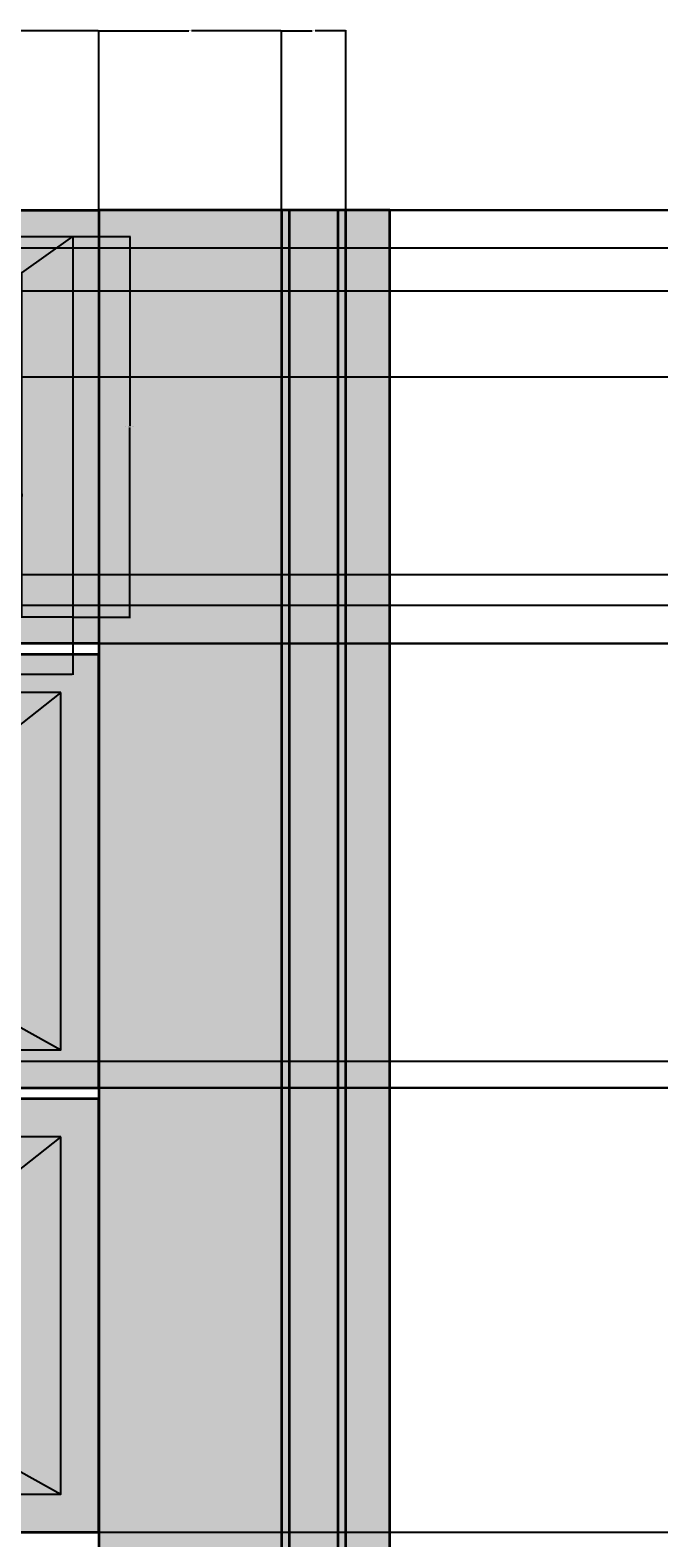
# Model space of a CAD drawing. Units: feet. Extents: x 1141 to 2858, y 751 to 1654.
# Tile 8 of 13: x 2096 to 2288, y 1195 to 1654. Entities that reach past the tile are written whole.
import ezdxf

# ---------------------------------------------------------------- set-up
doc = ezdxf.new("R2010")
doc.units = ezdxf.units.FT
for name, color, linetype, lineweight in [('A-ANNO-DIMS', 2, 'Continuous', 18), ('A-ELEV', 7, 'Continuous', 35), ('A-ELEV-PATT', 8, 'Continuous', 13), ('A-GLAZ', 4, 'Continuous', 25)]:
    doc.layers.add(name, color=color, linetype=linetype, lineweight=lineweight)
doc.styles.get("Standard").update_dxf_attribs({"font": 'arial.ttf'})
doc.dimstyles.get("Standard").update_dxf_attribs({"dimtxt": 0.18, "dimasz": 0.18, "dimexe": 0.18, "dimexo": 0.0625, "dimgap": 0.09, "dimtad": 0, "dimtih": 1, "dimtoh": 1, "dimdec": 1, "dimzin": 0, "dimdsep": 46, "dimlunit": 3, "dimtxsty": 'Standard', "dimcen": 0.09, "dimadec": 0, "dimazin": 0, "dimtfac": 1, "dimtdec": 1, "dimtofl": 0, "dimtmove": 0, "dimatfit": 3, "dimfxl": 1, "dimtolj": 1, "dimtzin": 0, "dimarcsym": 0})

# ---------------------------------------------------------------- blocks, each defined once
blk = doc.blocks.new('WIN-SIDE-A')
blk.add_line((63.09, 104.94), (78.57, 116.03))
blk.add_line((63.09, 104.94), (78.57, 116.03))
for points in [[(78.57, 0), (0, 0), (0, 116.03), (78.57, 116.03)], [(78.57, 0), (0, 0), (0, 116.03), (78.57, 116.03)], [(31.54, 104.94), (32.46, 104.94), (32.46, 0), (31.54, 0)], [(0, 37.61), (63.09, 37.61), (63.09, 36.79), (0, 36.79)]]:
    blk.add_lwpolyline(points, close=True)
for points in [[(63.09, 0), (63.09, 104.94), (0, 104.94)], [(63.09, 0), (63.09, 104.94), (0, 104.94)], [(31.54, 37.61), (31.54, 104.94), (32.46, 104.94), (32.46, 37.61)], [(31.54, 36.79), (0, 36.79), (0, 37.61), (31.54, 37.61)], [(32.46, 36.79), (32.46, 0), (31.54, 0), (31.54, 36.79)], [(32.46, 37.61), (63.09, 37.61), (63.09, 36.79), (32.46, 36.79)]]:
    blk.add_lwpolyline(points)
blk = doc.blocks.new('BALCONY-GLAZ-A')
for p, q in [((0, 108.84), (16.63, 95.74)), ((0, 108.84), (16.63, 95.74)), ((266.62, 95.74), (273.67, 108.84)), ((266.62, 95.74), (273.67, 108.84)), ((16.63, 95.74), (16.63, 9.29)), ((16.63, 95.74), (266.62, 95.74)), ((16.63, 95.74), (16.63, 9.29)), ((16.63, 95.74), (266.62, 95.74)), ((266.62, 95.74), (266.62, 9.19)), ((266.62, 95.74), (266.62, 9.19)), ((16.63, 9.29), (0, 0)), ((16.63, 9.29), (0, 0)), ((16.63, 9.29), (266.62, 9.29)), ((16.63, 9.29), (266.62, 9.29)), ((266.62, 9.29), (273.67, 0)), ((266.62, 9.29), (273.67, 0))]:
    blk.add_line(p, q)
for points in [[(0, 108.84), (273.67, 108.84), (273.67, 0), (0, 0)], [(0, 108.84), (273.67, 108.84), (273.67, 0), (0, 0)], [(266.62, 9.19), (168.47, 9.19), (168.47, 95.74), (266.62, 95.74)], [(266.62, 9.19), (168.47, 9.19), (168.47, 95.74), (266.62, 95.74)]]:
    blk.add_lwpolyline(points, close=True)
blk = doc.blocks.new('*D14')
at = {"layer": 'A-ANNO-DIMS', "color": 0, "lineweight": -2, "transparency": 16777216}
for p, q in [((2109.48, 1591.47), (2127.01, 1591.47)), ((2126.83, 1591.29), (2126.83, 1533.64)), ((2126.83, 1475.62), (2126.83, 1533.27)), ((2109.48, 1475.44), (2127.01, 1475.44))]:
    blk.add_line(p, q, dxfattribs=at)
at = {"layer": 'A-ANNO-DIMS', "color": 0, "transparency": 16777216}
for points in [[(2126.8, 1591.29), (2126.86, 1591.29), (2126.83, 1591.47)], [(2126.8, 1475.62), (2126.86, 1475.62), (2126.83, 1475.44)]]:
    blk.add_solid(points, dxfattribs=at)
at = {"layer": 'Defpoints', "color": 0, "transparency": 16777216}
for p in [(2109.42, 1591.47), (2126.83, 1591.47), (2109.42, 1475.44)]:
    blk.add_point(p, dxfattribs=at)
at = {"layer": 'A-ANNO-DIMS', "color": 0, "transparency": 16777216, "insert": (2126.83, 1533.45), "char_height": 0.18, "attachment_point": 5}
blk.add_mtext('\\A1;SIDE WINDOW A 116 TYP.', dxfattribs=at)
blk = doc.blocks.new('*D15')
at = {"layer": 'A-ANNO-DIMS', "color": 0, "lineweight": -2, "transparency": 16777216}
for p, q in [((2030.85, 1475.38), (2030.85, 1457.85)), ((2109.42, 1475.38), (2109.42, 1457.85)), ((2031.03, 1458.03), (2069.61, 1458.03)), ((2109.24, 1458.03), (2070.66, 1458.03))]:
    blk.add_line(p, q, dxfattribs=at)
at = {"layer": 'A-ANNO-DIMS', "color": 0, "transparency": 16777216}
for points in [[(2031.03, 1458.06), (2031.03, 1458), (2030.85, 1458.03)], [(2109.24, 1458.06), (2109.24, 1458), (2109.42, 1458.03)]]:
    blk.add_solid(points, dxfattribs=at)
at = {"layer": 'Defpoints', "color": 0, "transparency": 16777216}
for p in [(2030.85, 1475.44), (2109.42, 1475.44), (2109.42, 1458.03)]:
    blk.add_point(p, dxfattribs=at)
at = {"layer": 'A-ANNO-DIMS', "color": 0, "transparency": 16777216, "insert": (2070.14, 1458.03), "char_height": 0.18, "attachment_point": 5}
blk.add_mtext('\\A1;79 TYP.', dxfattribs=at)
blk = doc.blocks.new('*D26')
at = {"layer": 'A-ANNO-DIMS', "color": 0, "lineweight": -2, "transparency": 16777216}
for p, q in [((2022.87, 1599.52), (2022.87, 1654.28)), ((2023.05, 1654.1), (2069.74, 1654.1)), ((2117.23, 1654.1), (2070.53, 1654.1)), ((2117.41, 1599.52), (2117.41, 1654.28))]:
    blk.add_line(p, q, dxfattribs=at)
at = {"layer": 'A-ANNO-DIMS', "color": 0, "transparency": 16777216}
for points in [[(2023.05, 1654.13), (2023.05, 1654.07), (2022.87, 1654.1)], [(2117.23, 1654.13), (2117.23, 1654.07), (2117.41, 1654.1)]]:
    blk.add_solid(points, dxfattribs=at)
at = {"layer": 'Defpoints', "color": 0, "transparency": 16777216}
for p in [(2117.41, 1654.1), (2022.87, 1599.45), (2117.41, 1599.45)]:
    blk.add_point(p, dxfattribs=at)
at = {"layer": 'A-ANNO-DIMS', "color": 0, "transparency": 16777216, "insert": (2070.14, 1654.1), "char_height": 0.18, "attachment_point": 5}
blk.add_mtext('\\A1;94.54', dxfattribs=at)
blk = doc.blocks.new('*D27')
at = {"layer": 'A-ANNO-DIMS', "color": 0, "lineweight": -2, "transparency": 16777216}
for p, q in [((2117.41, 1599.52), (2117.41, 1654.28)), ((2117.59, 1654.1), (2144.83, 1654.1)), ((2172.84, 1654.1), (2145.59, 1654.1)), ((2173.02, 1599.52), (2173.02, 1654.28))]:
    blk.add_line(p, q, dxfattribs=at)
at = {"layer": 'A-ANNO-DIMS', "color": 0, "transparency": 16777216}
for points in [[(2117.59, 1654.13), (2117.59, 1654.07), (2117.41, 1654.1)], [(2172.84, 1654.13), (2172.84, 1654.07), (2173.02, 1654.1)]]:
    blk.add_solid(points, dxfattribs=at)
at = {"layer": 'Defpoints', "color": 0, "transparency": 16777216}
for p in [(2173.02, 1654.1), (2117.41, 1599.45), (2173.02, 1599.45)]:
    blk.add_point(p, dxfattribs=at)
at = {"layer": 'A-ANNO-DIMS', "color": 0, "transparency": 16777216, "insert": (2145.21, 1654.1), "char_height": 0.18, "attachment_point": 5}
blk.add_mtext('\\A1;55.61', dxfattribs=at)
blk = doc.blocks.new('*D28')
at = {"layer": 'A-ANNO-DIMS', "color": 0, "lineweight": -2, "transparency": 16777216}
for p, q in [((2173.02, 1599.52), (2173.02, 1654.28)), ((2173.2, 1654.1), (2182.4, 1654.1)), ((2192.51, 1654.1), (2183.31, 1654.1)), ((2192.69, 1599.52), (2192.69, 1654.28))]:
    blk.add_line(p, q, dxfattribs=at)
at = {"layer": 'A-ANNO-DIMS', "color": 0, "transparency": 16777216}
for points in [[(2173.2, 1654.13), (2173.2, 1654.07), (2173.02, 1654.1)], [(2192.51, 1654.13), (2192.51, 1654.07), (2192.69, 1654.1)]]:
    blk.add_solid(points, dxfattribs=at)
at = {"layer": 'Defpoints', "color": 0, "transparency": 16777216}
for p in [(2192.69, 1654.1), (2173.02, 1599.45), (2192.69, 1599.45)]:
    blk.add_point(p, dxfattribs=at)
at = {"layer": 'A-ANNO-DIMS', "color": 0, "transparency": 16777216, "insert": (2182.85, 1654.1), "char_height": 0.18, "attachment_point": 5}
blk.add_mtext('\\A1;19.673', dxfattribs=at)
blk = doc.blocks.new('*D31')
at = {"layer": 'A-ANNO-DIMS', "color": 0, "lineweight": -2, "transparency": 16777216}
for p, q in [((2117.47, 1196.68), (2857.83, 1196.68)), ((2857.65, 1196.5), (2857.65, 1129.16)), ((2857.65, 1061.47), (2857.65, 1128.8)), ((2117.47, 1061.29), (2857.83, 1061.29))]:
    blk.add_line(p, q, dxfattribs=at)
at = {"layer": 'A-ANNO-DIMS', "color": 0, "transparency": 16777216}
for points in [[(2857.62, 1196.5), (2857.68, 1196.5), (2857.65, 1196.68)], [(2857.62, 1061.47), (2857.68, 1061.47), (2857.65, 1061.29)]]:
    blk.add_solid(points, dxfattribs=at)
at = {"layer": 'Defpoints', "color": 0, "transparency": 16777216}
for p in [(2117.41, 1196.68), (2857.65, 1196.68), (2117.41, 1061.29)]:
    blk.add_point(p, dxfattribs=at)
at = {"layer": 'A-ANNO-DIMS', "color": 0, "transparency": 16777216, "insert": (2857.65, 1128.98), "char_height": 0.18, "attachment_point": 5}
blk.add_mtext('\\A1;135.4', dxfattribs=at)
blk = doc.blocks.new('*D32')
at = {"layer": 'A-ANNO-DIMS', "color": 0, "lineweight": -2, "transparency": 16777216}
for p, q in [((2117.47, 1332.06), (2857.83, 1332.06)), ((2857.65, 1331.88), (2857.65, 1264.55)), ((2857.65, 1196.86), (2857.65, 1264.19)), ((2117.47, 1196.68), (2857.83, 1196.68))]:
    blk.add_line(p, q, dxfattribs=at)
at = {"layer": 'A-ANNO-DIMS', "color": 0, "transparency": 16777216}
for points in [[(2857.62, 1331.88), (2857.68, 1331.88), (2857.65, 1332.06)], [(2857.62, 1196.86), (2857.68, 1196.86), (2857.65, 1196.68)]]:
    blk.add_solid(points, dxfattribs=at)
at = {"layer": 'Defpoints', "color": 0, "transparency": 16777216}
for p in [(2117.41, 1332.06), (2857.65, 1332.06), (2117.41, 1196.68)]:
    blk.add_point(p, dxfattribs=at)
at = {"layer": 'A-ANNO-DIMS', "color": 0, "transparency": 16777216, "insert": (2857.65, 1264.37), "char_height": 0.18, "attachment_point": 5}
blk.add_mtext('\\A1;135.4', dxfattribs=at)
blk = doc.blocks.new('*D33')
at = {"layer": 'A-ANNO-DIMS', "color": 0, "lineweight": -2, "transparency": 16777216}
for p, q in [((2117.47, 1467.45), (2857.83, 1467.45)), ((2857.65, 1467.27), (2857.65, 1399.94)), ((2857.65, 1332.24), (2857.65, 1399.58)), ((2117.47, 1332.06), (2857.83, 1332.06))]:
    blk.add_line(p, q, dxfattribs=at)
at = {"layer": 'A-ANNO-DIMS', "color": 0, "transparency": 16777216}
for points in [[(2857.62, 1467.27), (2857.68, 1467.27), (2857.65, 1467.45)], [(2857.62, 1332.24), (2857.68, 1332.24), (2857.65, 1332.06)]]:
    blk.add_solid(points, dxfattribs=at)
at = {"layer": 'Defpoints', "color": 0, "transparency": 16777216}
for p in [(2117.41, 1467.45), (2857.65, 1467.45), (2117.41, 1332.06)]:
    blk.add_point(p, dxfattribs=at)
at = {"layer": 'A-ANNO-DIMS', "color": 0, "transparency": 16777216, "insert": (2857.65, 1399.76), "char_height": 0.18, "attachment_point": 5}
blk.add_mtext('\\A1;135.4', dxfattribs=at)
blk = doc.blocks.new('*D34')
at = {"layer": 'A-ANNO-DIMS', "color": 0, "lineweight": -2, "transparency": 16777216}
for p, q in [((2117.47, 1599.45), (2857.83, 1599.45)), ((2857.65, 1599.27), (2857.65, 1533.63)), ((2857.65, 1467.63), (2857.65, 1533.27)), ((2117.47, 1467.45), (2857.83, 1467.45))]:
    blk.add_line(p, q, dxfattribs=at)
at = {"layer": 'A-ANNO-DIMS', "color": 0, "transparency": 16777216}
for points in [[(2857.62, 1599.27), (2857.68, 1599.27), (2857.65, 1599.45)], [(2857.62, 1467.63), (2857.68, 1467.63), (2857.65, 1467.45)]]:
    blk.add_solid(points, dxfattribs=at)
at = {"layer": 'Defpoints', "color": 0, "transparency": 16777216}
for p in [(2117.41, 1599.45), (2857.65, 1599.45), (2117.41, 1467.45)]:
    blk.add_point(p, dxfattribs=at)
at = {"layer": 'A-ANNO-DIMS', "color": 0, "transparency": 16777216, "insert": (2857.65, 1533.45), "char_height": 0.18, "attachment_point": 5}
blk.add_mtext('\\A1;132', dxfattribs=at)
blk = doc.blocks.new('*D39')
at = {"layer": 'A-ANNO-DIMS', "color": 0, "lineweight": -2, "transparency": 16777216}
for p, q in [((2319.24, 1599.45), (1668.14, 1599.45)), ((1668.32, 1599.27), (1668.32, 1202.86)), ((1668.32, 806.08), (1668.32, 1202.49)), ((2319.24, 805.9), (1668.14, 805.9))]:
    blk.add_line(p, q, dxfattribs=at)
at = {"layer": 'A-ANNO-DIMS', "color": 0, "transparency": 16777216}
for points in [[(1668.29, 1599.27), (1668.35, 1599.27), (1668.32, 1599.45)], [(1668.29, 806.08), (1668.35, 806.08), (1668.32, 805.9)]]:
    blk.add_solid(points, dxfattribs=at)
at = {"layer": 'Defpoints', "color": 0, "transparency": 16777216}
for p in [(1668.32, 1599.45), (2319.3, 1599.45), (2319.3, 805.9)]:
    blk.add_point(p, dxfattribs=at)
at = {"layer": 'A-ANNO-DIMS', "color": 0, "transparency": 16777216, "insert": (1668.32, 1202.68), "char_height": 0.18, "attachment_point": 5}
blk.add_mtext('\\A1;793.6', dxfattribs=at)
blk = doc.blocks.new('*D48')
at = {"layer": 'A-ANNO-DIMS', "color": 0, "lineweight": -2, "transparency": 16777216}
for p, q in [((2330.82, 1479.03), (1668.14, 1479.03)), ((1668.32, 1478.85), (1668.32, 1473.42)), ((1668.32, 1467.63), (1668.32, 1473.06)), ((2319.24, 1467.45), (1668.14, 1467.45))]:
    blk.add_line(p, q, dxfattribs=at)
at = {"layer": 'A-ANNO-DIMS', "color": 0, "transparency": 16777216}
for points in [[(1668.29, 1478.85), (1668.35, 1478.85), (1668.32, 1479.03)], [(1668.29, 1467.63), (1668.35, 1467.63), (1668.32, 1467.45)]]:
    blk.add_solid(points, dxfattribs=at)
at = {"layer": 'Defpoints', "color": 0, "transparency": 16777216}
for p in [(1668.32, 1479.03), (2330.88, 1479.03), (2319.3, 1467.45)]:
    blk.add_point(p, dxfattribs=at)
at = {"layer": 'A-ANNO-DIMS', "color": 0, "transparency": 16777216, "insert": (1668.32, 1473.24), "char_height": 0.18, "attachment_point": 5}
blk.add_mtext('\\A1;11.58', dxfattribs=at)
blk = doc.blocks.new('*D49')
at = {"layer": 'A-ANNO-DIMS', "color": 0, "lineweight": -2, "transparency": 16777216}
for p, q in [((2347.45, 1488.33), (1668.14, 1488.33)), ((1668.32, 1488.15), (1668.32, 1483.86)), ((2330.82, 1479.03), (1668.14, 1479.03)), ((1668.32, 1479.21), (1668.32, 1483.5))]:
    blk.add_line(p, q, dxfattribs=at)
at = {"layer": 'A-ANNO-DIMS', "color": 0, "transparency": 16777216}
for points in [[(1668.29, 1488.15), (1668.35, 1488.15), (1668.32, 1488.33)], [(1668.29, 1479.21), (1668.35, 1479.21), (1668.32, 1479.03)]]:
    blk.add_solid(points, dxfattribs=at)
at = {"layer": 'Defpoints', "color": 0, "transparency": 16777216}
for p in [(1668.32, 1488.33), (2347.51, 1488.33), (2330.88, 1479.03)]:
    blk.add_point(p, dxfattribs=at)
at = {"layer": 'A-ANNO-DIMS', "color": 0, "transparency": 16777216, "insert": (1668.32, 1483.68), "char_height": 0.18, "attachment_point": 5}
blk.add_mtext('\\A1;9.293', dxfattribs=at)
blk = doc.blocks.new('*D50')
at = {"layer": 'A-ANNO-DIMS', "color": 0, "lineweight": -2, "transparency": 16777216}
for p, q in [((2356.58, 1548.54), (1668.14, 1548.54)), ((1668.32, 1548.36), (1668.32, 1518.62)), ((1668.32, 1488.51), (1668.32, 1518.25)), ((2347.45, 1488.33), (1668.14, 1488.33))]:
    blk.add_line(p, q, dxfattribs=at)
at = {"layer": 'A-ANNO-DIMS', "color": 0, "transparency": 16777216}
for points in [[(1668.29, 1548.36), (1668.35, 1548.36), (1668.32, 1548.54)], [(1668.29, 1488.51), (1668.35, 1488.51), (1668.32, 1488.33)]]:
    blk.add_solid(points, dxfattribs=at)
at = {"layer": 'Defpoints', "color": 0, "transparency": 16777216}
for p in [(1668.32, 1548.54), (2356.64, 1548.54), (2347.51, 1488.33)]:
    blk.add_point(p, dxfattribs=at)
at = {"layer": 'A-ANNO-DIMS', "color": 0, "transparency": 16777216, "insert": (1668.32, 1518.43), "char_height": 0.18, "attachment_point": 5}
blk.add_mtext('\\A1;60.22', dxfattribs=at)
blk = doc.blocks.new('*D51')
at = {"layer": 'A-ANNO-DIMS', "color": 0, "lineweight": -2, "transparency": 16777216}
for p, q in [((2347.45, 1574.77), (1668.14, 1574.77)), ((1668.32, 1574.59), (1668.32, 1561.84)), ((1668.32, 1548.72), (1668.32, 1561.47)), ((2356.58, 1548.54), (1668.14, 1548.54))]:
    blk.add_line(p, q, dxfattribs=at)
at = {"layer": 'A-ANNO-DIMS', "color": 0, "transparency": 16777216}
for points in [[(1668.29, 1574.59), (1668.35, 1574.59), (1668.32, 1574.77)], [(1668.29, 1548.72), (1668.35, 1548.72), (1668.32, 1548.54)]]:
    blk.add_solid(points, dxfattribs=at)
at = {"layer": 'Defpoints', "color": 0, "transparency": 16777216}
for p in [(1668.32, 1574.77), (2347.51, 1574.77), (2356.64, 1548.54)]:
    blk.add_point(p, dxfattribs=at)
at = {"layer": 'A-ANNO-DIMS', "color": 0, "transparency": 16777216, "insert": (1668.32, 1561.66), "char_height": 0.18, "attachment_point": 5}
blk.add_mtext('\\A1;26.23', dxfattribs=at)
blk = doc.blocks.new('*D52')
at = {"layer": 'A-ANNO-DIMS', "color": 0, "lineweight": -2, "transparency": 16777216}
for p, q in [((2330.82, 1587.87), (1668.14, 1587.87)), ((1668.32, 1587.69), (1668.32, 1581.5)), ((1668.32, 1574.95), (1668.32, 1581.14)), ((2347.45, 1574.77), (1668.14, 1574.77))]:
    blk.add_line(p, q, dxfattribs=at)
at = {"layer": 'A-ANNO-DIMS', "color": 0, "transparency": 16777216}
for points in [[(1668.29, 1587.69), (1668.35, 1587.69), (1668.32, 1587.87)], [(1668.29, 1574.95), (1668.35, 1574.95), (1668.32, 1574.77)]]:
    blk.add_solid(points, dxfattribs=at)
at = {"layer": 'Defpoints', "color": 0, "transparency": 16777216}
for p in [(1668.32, 1587.87), (2330.88, 1587.87), (2347.51, 1574.77)]:
    blk.add_point(p, dxfattribs=at)
at = {"layer": 'A-ANNO-DIMS', "color": 0, "transparency": 16777216, "insert": (1668.32, 1581.32), "char_height": 0.18, "attachment_point": 5}
blk.add_mtext('\\A1;13.102', dxfattribs=at)
blk = doc.blocks.new('*D53')
at = {"layer": 'A-ANNO-DIMS', "color": 0, "lineweight": -2, "transparency": 16777216}
for p, q in [((2319.24, 1599.45), (1668.14, 1599.45)), ((1668.32, 1599.27), (1668.32, 1593.84)), ((1668.32, 1588.05), (1668.32, 1593.48)), ((2330.82, 1587.87), (1668.14, 1587.87))]:
    blk.add_line(p, q, dxfattribs=at)
at = {"layer": 'A-ANNO-DIMS', "color": 0, "transparency": 16777216}
for points in [[(1668.29, 1599.27), (1668.35, 1599.27), (1668.32, 1599.45)], [(1668.29, 1588.05), (1668.35, 1588.05), (1668.32, 1587.87)]]:
    blk.add_solid(points, dxfattribs=at)
at = {"layer": 'Defpoints', "color": 0, "transparency": 16777216}
for p in [(1668.32, 1599.45), (2319.3, 1599.45), (2330.88, 1587.87)]:
    blk.add_point(p, dxfattribs=at)
at = {"layer": 'A-ANNO-DIMS', "color": 0, "transparency": 16777216, "insert": (1668.32, 1593.66), "char_height": 0.18, "attachment_point": 5}
blk.add_mtext('\\A1;11.58', dxfattribs=at)
blk = doc.blocks.new('*D54')
at = {"layer": 'A-ANNO-DIMS', "color": 0, "lineweight": -2, "transparency": 16777216}
for p, q in [((2327.22, 1340.05), (1668.14, 1340.05)), ((1668.32, 1339.87), (1668.32, 1336.24)), ((2319.24, 1332.06), (1668.14, 1332.06)), ((1668.32, 1332.24), (1668.32, 1335.88))]:
    blk.add_line(p, q, dxfattribs=at)
at = {"layer": 'A-ANNO-DIMS', "color": 0, "transparency": 16777216}
for points in [[(1668.29, 1339.87), (1668.35, 1339.87), (1668.32, 1340.05)], [(1668.29, 1332.24), (1668.35, 1332.24), (1668.32, 1332.06)]]:
    blk.add_solid(points, dxfattribs=at)
at = {"layer": 'Defpoints', "color": 0, "transparency": 16777216}
for p in [(1668.32, 1340.05), (2327.29, 1340.05), (2319.3, 1332.06)]:
    blk.add_point(p, dxfattribs=at)
at = {"layer": 'A-ANNO-DIMS', "color": 0, "transparency": 16777216, "insert": (1668.32, 1336.06), "char_height": 0.18, "attachment_point": 5}
blk.add_mtext('\\A1;7.986', dxfattribs=at)

msp = doc.modelspace()

# ---------------------------------------------------------------- hatches: boundary and pattern name
at = {"layer": 'A-ELEV-PATT'}
h = msp.add_hatch(color=256, dxfattribs=at)
h.dxf.hatch_style = 1
h.paths.add_polyline_path([(2206.032, 1599.4527), (2192.689, 1599.4527), (2192.689, 919.339), (2206.032, 919.339)])
h.paths.add_polyline_path([(2190.2416, 1599.4527), (2175.463, 1599.4527), (2175.463, 919.339), (2190.2416, 919.339)])
h.paths.add_polyline_path([(2173.0156, 1599.4527), (2117.407, 1599.4527), (2117.407, 919.339), (2173.0156, 919.339)])
h.paths.add_polyline_path([(2022.8666, 1057.9008), (1726.032, 1057.9008), (1726.032, 925.9008), (2022.8666, 925.9008)])
h.paths.add_polyline_path([(1737.6123, 937.4811), (1737.6123, 1046.3205), (2011.2863, 1046.3205), (2011.2863, 937.4811)], flags=16)
h.paths.add_polyline_path([(1754.2423, 946.7736), (1754.2423, 1033.2183), (2004.2323, 1033.2183), (2004.2323, 946.7736), (2004.3069, 946.6754), (1906.0824, 946.6754)], flags=0)
h.paths.add_polyline_path([(1900.5421, 946.7736), (1857.5566, 946.7736), (1857.5566, 1033.2183), (1900.5421, 1033.2183)], flags=0)
h.paths.add_polyline_path([(1910.8368, 951.4297), (1910.8368, 1022.7957), (1999.478, 1022.7957), (1999.478, 951.4297)], flags=0)
h.paths.add_polyline_path([(1930.8039, 951.4297), (1930.8039, 1022.7957), (1932.373, 1022.7957), (1932.373, 951.4297)], flags=0)
h.paths.add_polyline_path([(1851.6414, 946.7736), (1826.5664, 946.7736), (1826.5664, 967.8234), (1793.4402, 967.8234), (1793.4402, 946.7736), (1790.4043, 946.7736), (1790.4043, 967.8234), (1754.2423, 967.8234), (1754.2423, 970.4796), (1790.4043, 970.4796), (1790.4043, 1033.2183), (1793.4402, 1033.2183), (1793.4402, 970.4796), (1826.5664, 970.4796), (1826.5664, 1033.2183), (1851.6414, 1033.2183)], flags=0)
h.paths.add_polyline_path([(1954.3728, 951.4297), (1954.3728, 1022.7957), (1955.9419, 1022.7957), (1955.9419, 951.4297)], flags=0)
h.paths.add_polyline_path([(1977.7327, 951.4297), (1977.7327, 1022.7957), (1979.3018, 1022.7957), (1979.3018, 951.4297)], flags=0)
h.paths.add_polyline_path([(2022.8666, 1193.2888), (1726.032, 1193.2888), (1726.032, 1061.2888), (2022.8666, 1061.2888)])
h.paths.add_polyline_path([(1737.6123, 1072.869), (1737.6123, 1181.7085), (2011.2863, 1181.7085), (2011.2863, 1072.869)], flags=16)
h.paths.add_polyline_path([(1754.2423, 1082.1616), (1754.2423, 1168.6063), (2004.2323, 1168.6063), (2004.2323, 1082.1616), (2004.3069, 1082.0634), (1906.0824, 1082.0634)], flags=0)
h.paths.add_polyline_path([(1900.5421, 1082.1616), (1857.5566, 1082.1616), (1857.5566, 1168.6063), (1900.5421, 1168.6063)], flags=0)
h.paths.add_polyline_path([(1910.8368, 1086.8177), (1910.8368, 1158.1837), (1999.478, 1158.1837), (1999.478, 1086.8177)], flags=0)
h.paths.add_polyline_path([(1930.8039, 1086.8177), (1930.8039, 1158.1837), (1932.373, 1158.1837), (1932.373, 1086.8177)], flags=0)
h.paths.add_polyline_path([(1851.6414, 1082.1616), (1826.5664, 1082.1616), (1826.5664, 1103.2114), (1793.4402, 1103.2114), (1793.4402, 1082.1616), (1790.4043, 1082.1616), (1790.4043, 1103.2114), (1754.2423, 1103.2114), (1754.2423, 1105.8676), (1790.4043, 1105.8676), (1790.4043, 1168.6063), (1793.4402, 1168.6063), (1793.4402, 1105.8676), (1826.5664, 1105.8676), (1826.5664, 1168.6063), (1851.6414, 1168.6063)], flags=0)
h.paths.add_polyline_path([(1954.3728, 1086.8177), (1954.3728, 1158.1837), (1955.9419, 1158.1837), (1955.9419, 1086.8177)], flags=0)
h.paths.add_polyline_path([(1977.7327, 1086.8177), (1977.7327, 1158.1837), (1979.3018, 1158.1837), (1979.3018, 1086.8177)], flags=0)
h.paths.add_polyline_path([(2022.8666, 1599.4527), (1726.032, 1599.4527), (1726.032, 1467.4527), (2022.8666, 1467.4527)])
h.paths.add_polyline_path([(2011.2863, 1479.033), (1737.6123, 1479.033), (1737.6123, 1587.8725), (2011.2863, 1587.8725)], flags=16)
h.paths.add_polyline_path([(2004.2323, 1488.3255), (1754.2423, 1488.3255), (1754.2423, 1574.7702), (2004.2323, 1574.7702)], flags=0)
h.paths.add_polyline_path([(1829.1345, 1544.6458), (1914.1177, 1544.6458), (1914.1177, 1539.5463), (1830.9097, 1539.5463), (1831.6817, 1537.3286), (1914.1177, 1537.3286), (1914.1177, 1532.2291), (1833.4569, 1532.2291), (1834.229, 1530.0113), (1914.1177, 1530.0113), (1914.1177, 1524.9118), (1836.0042, 1524.9118), (1836.7762, 1522.694), (1914.1177, 1522.694), (1914.1177, 1517.5946), (1838.5514, 1517.5946), (1839.3235, 1515.3768), (1914.1177, 1515.3768), (1914.1177, 1510.2773), (1841.0987, 1510.2773), (1841.8707, 1508.0595), (1914.1177, 1508.0595), (1914.1177, 1502.9601), (1843.6459, 1502.9601), (1844.4179, 1500.7423), (1914.1177, 1500.7423), (1914.1177, 1495.6428), (1846.1931, 1495.6428), (1846.9652, 1493.425), (1914.1177, 1493.425), (1914.1177, 1488.3255), (1848.6593, 1488.3255), (1848.6593, 1488.5583)], flags=0)
h.paths.add_polyline_path([(2117.407, 1464.0647), (1820.5724, 1464.0647), (1820.5724, 1332.0647), (2117.407, 1332.0647)])
h.paths.add_polyline_path([(2105.8267, 1452.4845), (2105.8267, 1343.645), (1832.1527, 1343.645), (1832.1527, 1452.4845)], flags=16)
h.paths.add_polyline_path([(2089.1967, 1439.3822), (2089.1967, 1352.9376), (1937.3566, 1352.9376), (1937.3566, 1352.8393), (1839.1321, 1352.8393), (1839.2067, 1352.9376), (1839.2067, 1439.3822), (1937.3566, 1439.3822)], flags=0)
h.paths.add_polyline_path([(2016.8727, 1439.3822), (2016.8727, 1376.6436), (2049.9988, 1376.6436), (2049.9988, 1439.3822), (2053.0347, 1439.3822), (2053.0347, 1376.6436), (2089.1967, 1376.6436), (2089.1967, 1373.9873), (2053.0347, 1373.9873), (2053.0347, 1352.9376), (2049.9988, 1352.9376), (2049.9988, 1373.9873), (2016.8727, 1373.9873), (2016.8727, 1352.9376), (1991.7976, 1352.9376), (1991.7976, 1439.3822)], flags=0)
h.paths.add_polyline_path([(1985.8824, 1439.3822), (1985.8824, 1352.9376), (1942.8969, 1352.9376), (1942.8969, 1439.3822)], flags=0)
h.paths.add_polyline_path([(1932.6022, 1428.9596), (1932.6022, 1357.5937), (1843.961, 1357.5937), (1843.961, 1428.9596)], flags=0)
h.paths.add_polyline_path([(1912.6351, 1428.9596), (1912.6351, 1357.5937), (1911.066, 1357.5937), (1911.066, 1428.9596)], flags=0)
h.paths.add_polyline_path([(1889.0662, 1428.9596), (1889.0662, 1357.5937), (1887.4971, 1357.5937), (1887.4971, 1428.9596)], flags=0)
h.paths.add_polyline_path([(1865.7063, 1428.9596), (1865.7063, 1357.5937), (1864.1372, 1357.5937), (1864.1372, 1428.9596)], flags=0)
h.paths.add_polyline_path([(2117.407, 1328.6768), (1820.5724, 1328.6768), (1820.5724, 1196.6768), (2117.407, 1196.6768)])
h.paths.add_polyline_path([(2105.8267, 1317.0965), (2105.8267, 1208.257), (1832.1527, 1208.257), (1832.1527, 1317.0965)], flags=16)
h.paths.add_polyline_path([(2089.1967, 1303.9943), (2089.1967, 1217.5496), (1937.3566, 1217.5496), (1937.3566, 1217.4513), (1839.1321, 1217.4513), (1839.2067, 1217.5496), (1839.2067, 1303.9943), (1937.3566, 1303.9943)], flags=0)
h.paths.add_polyline_path([(2016.8727, 1303.9943), (2016.8727, 1241.2556), (2049.9988, 1241.2556), (2049.9988, 1303.9943), (2053.0347, 1303.9943), (2053.0347, 1241.2556), (2089.1967, 1241.2556), (2089.1967, 1238.5993), (2053.0347, 1238.5993), (2053.0347, 1217.5496), (2049.9988, 1217.5496), (2049.9988, 1238.5993), (2016.8727, 1238.5993), (2016.8727, 1217.5496), (1991.7976, 1217.5496), (1991.7976, 1303.9943)], flags=0)
h.paths.add_polyline_path([(1985.8824, 1303.9943), (1985.8824, 1217.5496), (1942.8969, 1217.5496), (1942.8969, 1303.9943)], flags=0)
h.paths.add_polyline_path([(1932.6022, 1293.5716), (1932.6022, 1222.2057), (1843.961, 1222.2057), (1843.961, 1293.5716)], flags=0)
h.paths.add_polyline_path([(1912.6351, 1293.5716), (1912.6351, 1222.2057), (1911.066, 1222.2057), (1911.066, 1293.5716)], flags=0)
h.paths.add_polyline_path([(1889.0662, 1293.5716), (1889.0662, 1222.2057), (1887.4971, 1222.2057), (1887.4971, 1293.5716)], flags=0)
h.paths.add_polyline_path([(1865.7063, 1293.5716), (1865.7063, 1222.2057), (1864.1372, 1222.2057), (1864.1372, 1293.5716)], flags=0)
h.paths.add_polyline_path([(2206.032, 917.3598), (2027.2589, 917.3598), (2027.2589, 805.9008), (2206.032, 805.9008)])
h.paths.add_polyline_path([(1852.1771, 917.3598), (1726.032, 917.3598), (1726.032, 805.9008), (1852.1771, 805.9008)])
h.paths.add_polyline_path([(2063.3101, 1580.3829), (2093.938, 1580.3829), (2093.938, 1513.0494), (2063.3101, 1513.0494)])
h.paths.add_polyline_path([(2063.3101, 1580.3829), (2093.938, 1580.3829), (2093.938, 1513.0494), (2063.3101, 1513.0494)])
h = msp.add_hatch(color=256, dxfattribs=at)
h.dxf.hatch_style = 1
h.paths.add_polyline_path([(2011.2863, 1587.8725), (1737.6123, 1587.8725), (1754.2423, 1574.7702), (2004.2323, 1574.7702)])
h.paths.add_polyline_path([(1754.2423, 1574.7702), (1737.6123, 1587.8725), (1737.6123, 1479.033), (1754.2423, 1488.3255)])
h.paths.add_polyline_path([(2011.2863, 1587.8725), (2004.2323, 1574.7702), (2004.2323, 1488.3255), (2011.2863, 1479.033)])
h.paths.add_polyline_path([(2004.2323, 1488.3255), (1754.2423, 1488.3255), (1737.6123, 1479.033), (2011.2863, 1479.033)])
h.paths.add_polyline_path([(2105.8267, 1452.4845), (1832.1527, 1452.4845), (1839.2067, 1439.3822), (1937.3566, 1439.3822), (2089.1967, 1439.3822)])
h.paths.add_polyline_path([(1839.2067, 1439.3822), (1832.1527, 1452.4845), (1832.1527, 1343.645), (1839.2067, 1352.9376)])
h.paths.add_polyline_path([(2105.8267, 1452.4845), (2089.1967, 1439.3822), (2089.1967, 1352.9376), (2105.8267, 1343.645)])
h.paths.add_polyline_path([(2089.1967, 1352.9376), (1937.3566, 1352.9376), (1937.3566, 1352.8393), (1839.1321, 1352.8393), (1832.1527, 1343.645), (2105.8267, 1343.645)])
h.paths.add_polyline_path([(1942.8969, 1439.3822), (1937.3566, 1439.3822), (1937.3566, 1352.9376), (1942.8969, 1352.9376)])
h.paths.add_polyline_path([(1991.7976, 1439.3822), (1985.8824, 1439.3822), (1985.8824, 1352.9376), (1991.7976, 1352.9376)])
h.paths.add_polyline_path([(2109.4211, 1591.4669), (2030.8524, 1591.4669), (2030.8524, 1580.3829), (2093.938, 1580.3829)])
h.paths.add_polyline_path([(2109.4211, 1591.4669), (2093.938, 1580.3829), (2093.938, 1475.4386), (2109.4211, 1475.4386)])
h.paths.add_polyline_path([(1991.7976, 1303.9943), (1985.8824, 1303.9943), (1985.8824, 1217.5496), (1991.7976, 1217.5496)])
h.paths.add_polyline_path([(1942.8969, 1303.9943), (1937.3566, 1303.9943), (1937.3566, 1217.5496), (1942.8969, 1217.5496)])
h.paths.add_polyline_path([(2105.8267, 1317.0965), (1832.1527, 1317.0965), (1839.2067, 1303.9943), (1937.3566, 1303.9943), (2089.1967, 1303.9943)])
h.paths.add_polyline_path([(1839.2067, 1303.9943), (1832.1527, 1317.0965), (1832.1527, 1208.257), (1839.2067, 1217.5496)])
h.paths.add_polyline_path([(2089.1967, 1217.5496), (1937.3566, 1217.5496), (1937.3566, 1217.4513), (1839.1321, 1217.4513), (1832.1527, 1208.257), (2105.8267, 1208.257)])
h.paths.add_polyline_path([(2105.8267, 1317.0965), (2089.1967, 1303.9943), (2089.1967, 1217.5496), (2105.8267, 1208.257)])
h.paths.add_polyline_path([(1754.2423, 1168.6063), (1737.6123, 1181.7085), (1737.6123, 1072.869), (1754.2423, 1082.1616)])
h.paths.add_polyline_path([(2011.2863, 1181.7085), (1737.6123, 1181.7085), (1754.2423, 1168.6063), (2004.2323, 1168.6063)])
h.paths.add_polyline_path([(2011.2863, 1181.7085), (2004.2323, 1168.6063), (2004.2323, 1082.1616), (2011.2863, 1072.869)])
h.paths.add_polyline_path([(2004.3069, 1082.0634), (1906.0824, 1082.0634), (1754.2423, 1082.1616), (1737.6123, 1072.869), (2011.2863, 1072.869)])
h.paths.add_polyline_path([(1906.0824, 1168.6063), (1900.5421, 1168.6063), (1900.5421, 1082.1616), (1906.0824, 1082.1616)])
h.paths.add_polyline_path([(1857.5566, 1168.6063), (1851.6414, 1168.6063), (1851.6414, 1082.1616), (1857.5566, 1082.1616)])
h.paths.add_polyline_path([(1906.0824, 1033.2183), (1900.5421, 1033.2183), (1900.5421, 946.7736), (1906.0824, 946.7736)])
h.paths.add_polyline_path([(1857.5566, 1033.2183), (1851.6414, 1033.2183), (1851.6414, 946.7736), (1857.5566, 946.7736)])
h.paths.add_polyline_path([(1754.2423, 1033.2183), (1737.6123, 1046.3205), (1737.6123, 937.4811), (1754.2423, 946.7736)])
h.paths.add_polyline_path([(2011.2863, 1046.3205), (1737.6123, 1046.3205), (1754.2423, 1033.2183), (2004.2323, 1033.2183)])
h.paths.add_polyline_path([(2011.2863, 1046.3205), (2004.2323, 1033.2183), (2004.2323, 946.7736), (2011.2863, 937.4811)])
h.paths.add_polyline_path([(2004.3069, 946.6754), (1906.0824, 946.6754), (1754.2423, 946.7736), (1737.6123, 937.4811), (2011.2863, 937.4811)])
h.paths.add_polyline_path([(2175.463, 1599.4527), (2173.0156, 1599.4527), (2173.0156, 919.339), (2175.463, 919.339)])
h = msp.add_hatch(color=256, dxfattribs=at)
h.dxf.hatch_style = 1
h.paths.add_polyline_path([(2117.407, 1599.4527), (2022.8666, 1599.4527), (2022.8666, 1467.4527), (2117.407, 1467.4527)])
h.paths.add_polyline_path([(2109.4211, 1591.4669), (2109.4211, 1475.4386), (2030.8524, 1475.4386), (2030.8524, 1591.4669)], flags=16)
h.paths.add_polyline_path([(2093.938, 1580.3829), (2093.938, 1512.23), (2063.3101, 1512.23), (2063.3101, 1475.4386), (2062.3952, 1475.4386), (2062.3952, 1512.23), (2030.8524, 1512.23), (2030.8524, 1513.0494), (2062.3952, 1513.0494), (2062.3952, 1580.3829), (2063.3101, 1580.3829)], flags=0)
h = msp.add_hatch(color=256, dxfattribs=at)
h.dxf.hatch_style = 1
h.paths.add_polyline_path([(2192.689, 1599.4527), (2190.2416, 1599.4527), (2190.2416, 919.339), (2192.689, 919.339)])
h = msp.add_hatch(color=256, dxfattribs=at)
h.dxf.hatch_style = 1
h.paths.add_polyline_path([(2062.3952, 1580.3829), (2030.8524, 1580.3829), (2030.8524, 1513.0494), (2062.3952, 1513.0494)])
h.paths.add_polyline_path([(2093.938, 1580.3829), (2063.3101, 1580.3829), (2063.3101, 1513.0494), (2093.938, 1513.0494)])
h.paths.add_polyline_path([(2093.938, 1512.23), (2063.3101, 1512.23), (2063.3101, 1475.4386), (2093.938, 1475.4386)])
h.paths.add_polyline_path([(2062.3952, 1512.23), (2030.8524, 1512.23), (2030.8524, 1475.4386), (2062.3952, 1475.4386)])
h.paths.add_polyline_path([(1780.1289, 1444.9949), (1749.501, 1444.9949), (1749.501, 1377.6615), (1780.1289, 1377.6615)])
h.paths.add_polyline_path([(1812.5866, 1444.9949), (1781.0438, 1444.9949), (1781.0438, 1377.6615), (1812.5866, 1377.6615)])
h.paths.add_polyline_path([(1812.5866, 1376.842), (1781.0438, 1376.842), (1781.0438, 1340.0506), (1812.5866, 1340.0506)])
h.paths.add_polyline_path([(1780.1289, 1376.842), (1749.501, 1376.842), (1749.501, 1340.0506), (1780.1289, 1340.0506)])
h.paths.add_polyline_path([(2105.8267, 1452.4845), (1832.1527, 1452.4845), (1832.1527, 1343.645), (1839.2067, 1352.9376), (1839.2067, 1439.3822), (1937.3566, 1439.3822), (1937.3566, 1352.9376), (1942.8969, 1352.9376), (1942.8969, 1439.3822), (1985.8824, 1439.3822), (1985.8824, 1352.9376), (1991.7976, 1352.9376), (1991.7976, 1439.3822), (2016.8727, 1439.3822), (2016.8727, 1376.6436), (2049.9988, 1376.6436), (2049.9988, 1439.3822), (2053.0347, 1439.3822), (2053.0347, 1376.6436), (2089.1967, 1376.6436), (2089.1967, 1373.9873), (2053.0347, 1373.9873), (2053.0347, 1352.9376), (2049.9988, 1352.9376), (1937.3566, 1352.9376), (1937.3566, 1352.8393), (1839.1321, 1352.8393), (1832.1527, 1343.645), (2105.8267, 1343.645)])
h.paths.add_polyline_path([(2049.9988, 1373.9873), (2016.8727, 1373.9873), (2016.8727, 1352.9376), (2049.9988, 1352.9376)], flags=17)
h.paths.add_polyline_path([(1780.1289, 1309.6069), (1749.501, 1309.6069), (1749.501, 1242.2735), (1780.1289, 1242.2735)])
h.paths.add_polyline_path([(1812.5866, 1309.6069), (1781.0438, 1309.6069), (1781.0438, 1242.2735), (1812.5866, 1242.2735)])
h.paths.add_polyline_path([(1812.5866, 1241.454), (1781.0438, 1241.454), (1781.0438, 1204.6626), (1812.5866, 1204.6626)])
h.paths.add_polyline_path([(1780.1289, 1241.454), (1749.501, 1241.454), (1749.501, 1204.6626), (1780.1289, 1204.6626)])
h.paths.add_polyline_path([(2049.9988, 1303.9943), (2016.8727, 1303.9943), (2016.8727, 1241.2556), (2049.9988, 1241.2556)])
h.paths.add_polyline_path([(2089.1967, 1303.9943), (2053.0347, 1303.9943), (2053.0347, 1241.2556), (2089.1967, 1241.2556)])
h.paths.add_polyline_path([(2089.1967, 1238.5993), (2053.0347, 1238.5993), (2053.0347, 1217.5496), (2089.1967, 1217.5496)])
h.paths.add_polyline_path([(2049.9988, 1238.5993), (2016.8727, 1238.5993), (2016.8727, 1217.5496), (2049.9988, 1217.5496)])
h.paths.add_polyline_path([(2062.3952, 1174.219), (2030.8524, 1174.219), (2030.8524, 1106.8855), (2062.3952, 1106.8855)])
h.paths.add_polyline_path([(2093.938, 1174.219), (2063.3101, 1174.219), (2063.3101, 1106.8855), (2093.938, 1106.8855)])
h.paths.add_polyline_path([(2093.938, 1106.066), (2063.3101, 1106.066), (2063.3101, 1069.2747), (2093.938, 1069.2747)])
h.paths.add_polyline_path([(2062.3952, 1106.066), (2030.8524, 1106.066), (2030.8524, 1069.2747), (2062.3952, 1069.2747)])
h.paths.add_polyline_path([(1906.0824, 1168.6063), (2004.2323, 1168.6063), (2011.2863, 1181.7085), (1737.6123, 1181.7085), (1737.6123, 1072.869), (2011.2863, 1072.869), (2004.3069, 1082.0634), (1906.0824, 1082.0634)])
h.paths.add_polyline_path([(1790.4043, 1168.6063), (1793.4402, 1168.6063), (1793.4402, 1105.8676), (1826.5664, 1105.8676), (1826.5664, 1168.6063), (1851.6414, 1168.6063), (1851.6414, 1082.1616), (1826.5664, 1082.1616), (1826.5664, 1103.2114), (1793.4402, 1103.2114), (1793.4402, 1082.1616), (1790.4043, 1082.1616), (1790.4043, 1103.2114), (1754.2423, 1103.2114), (1754.2423, 1105.8676), (1790.4043, 1105.8676)], flags=16)
h.paths.add_polyline_path([(1857.5566, 1168.6063), (1900.5421, 1168.6063), (1900.5421, 1082.1616), (1857.5566, 1082.1616)], flags=16)

# ---------------------------------------------------------------- linework, layer by layer
at = {"layer": 'A-ELEV'}
for points in [[(2117.407, 1467.4527), (2022.8666, 1467.4527), (2022.8666, 1599.4527), (2117.407, 1599.4527)], [(2117.407, 1467.4527), (2022.8666, 1467.4527), (2022.8666, 1599.4527), (2117.407, 1599.4527)], [(2117.407, 1464.0647), (1820.5724, 1464.0647), (1820.5724, 1332.0647), (2117.407, 1332.0647)], [(2117.407, 1464.0647), (1820.5724, 1464.0647), (1820.5724, 1332.0647), (2117.407, 1332.0647)], [(2117.407, 1328.6768), (1820.5724, 1328.6768), (1820.5724, 1196.6768), (2117.407, 1196.6768)], [(2117.407, 1328.6768), (1820.5724, 1328.6768), (1820.5724, 1196.6768), (2117.407, 1196.6768)]]:
    msp.add_lwpolyline(points, close=True, dxfattribs=at)
for points in [[(2206.032, 919.339), (2206.032, 1599.4527), (2117.407, 1599.4527), (2117.407, 919.339)], [(2206.032, 919.339), (2206.032, 1599.4527), (2117.407, 1599.4527), (2117.407, 919.339)], [(2175.463, 919.339), (2175.463, 1599.4527), (2173.0156, 1599.4527), (2173.0156, 919.339)], [(2192.689, 919.339), (2192.689, 1599.4527), (2190.2416, 1599.4527), (2190.2416, 919.339)], [(2192.689, 919.339), (2192.689, 1599.4527), (2190.2416, 1599.4527), (2190.2416, 919.339)], [(2192.689, 919.339), (2192.689, 1599.4527), (2190.2416, 1599.4527), (2190.2416, 919.339)]]:
    msp.add_lwpolyline(points, dxfattribs=at)

# ---------------------------------------------------------------- block references
at = {"layer": 'A-GLAZ'}
msp.add_blockref('WIN-SIDE-A', (2030.852, 1475.439), dxfattribs=at)
at = {"layer": 'A-GLAZ', "extrusion": (0, 0, -1), "zscale": -1}
for p in [(-2105.827, 1343.6449), (-2105.827, 1208.257)]:
    msp.add_blockref('BALCONY-GLAZ-A', p, dxfattribs=at)

# ---------------------------------------------------------------- dimensions: what is measured, and where the dimension line sits
at = {"layer": 'A-ANNO-DIMS'}
for base, p1, p2, override, picture, middle in [((2117.407, 1654.1027), (2022.8666, 1599.4527), (2117.407, 1599.4527), {"dimdec": 2, "dimlfac": 1, "dimrnd": 0, "dimzin": 0, "dimdsep": 46, "dimlunit": 2}, '*D26', (2070.1368, 1654.1027)), ((2173.0156, 1654.1027), (2117.407, 1599.4527), (2173.0156, 1599.4527), {"dimdec": 2, "dimlfac": 1, "dimrnd": 0, "dimzin": 0, "dimdsep": 46, "dimlunit": 2}, '*D27', (2145.2113, 1654.1027)), ((2192.689, 1654.1027), (2173.0156, 1599.4527), (2192.689, 1599.4527), {"dimdec": 3, "dimlfac": 1, "dimrnd": 0, "dimzin": 0, "dimdsep": 46, "dimlunit": 2}, '*D28', (2182.8523, 1654.1027))]:
    dim = msp.add_linear_dim(base=base, p1=p1, p2=p2, dimstyle='Standard', override=override, dxfattribs=at)
    dim.commit()
    dim.dimension.update_dxf_attribs({"geometry": picture, "text_midpoint": middle})
for base, p1, p2, override, picture, middle in [((1668.3207, 1599.4527), (2319.3013, 805.9008), (2319.3013, 1599.4527), {"dimdec": 1, "dimlfac": 1, "dimrnd": 0, "dimzin": 0, "dimdsep": 46, "dimlunit": 2}, '*D39', (1668.3207, 1202.6768)), ((1668.3207, 1599.4527), (2330.8815, 1587.8725), (2319.3013, 1599.4527), {"dimdec": 2, "dimlfac": 1, "dimrnd": 0, "dimzin": 0, "dimdsep": 46, "dimlunit": 2}, '*D53', (1668.3207, 1593.6626)), ((2857.6489, 1599.4527), (2117.407, 1467.4527), (2117.407, 1599.4527), {"dimdec": 0, "dimlfac": 1, "dimrnd": 0, "dimzin": 0, "dimdsep": 46, "dimlunit": 2}, '*D34', (2857.6489, 1533.4527)), ((1668.3207, 1587.8725), (2347.5116, 1574.7702), (2330.8815, 1587.8725), {"dimdec": 3, "dimlfac": 1, "dimrnd": 0, "dimzin": 0, "dimdsep": 46, "dimlunit": 2}, '*D52', (1668.3207, 1581.3214)), ((1668.3207, 1574.7702), (2356.6424, 1548.5407), (2347.5116, 1574.7702), {"dimdec": 2, "dimlfac": 1, "dimrnd": 0, "dimzin": 0, "dimdsep": 46, "dimlunit": 2}, '*D51', (1668.3207, 1561.6555)), ((1668.3207, 1548.5407), (2347.5116, 1488.3255), (2356.6424, 1548.5407), {"dimdec": 2, "dimlfac": 1, "dimrnd": 0, "dimzin": 0, "dimdsep": 46, "dimlunit": 2}, '*D50', (1668.3207, 1518.4331)), ((1668.32065, 1488.32554), (2330.88152, 1479.03299), (2347.51155, 1488.32554), {"dimdec": 3, "dimlfac": 1, "dimrnd": 0, "dimzin": 0, "dimdsep": 46, "dimlunit": 2}, '*D49', (1668.32065, 1483.67926)), ((1668.3207, 1479.033), (2319.3013, 1467.4527), (2330.8815, 1479.033), {"dimdec": 2, "dimlfac": 1, "dimrnd": 0, "dimzin": 0, "dimdsep": 46, "dimlunit": 2}, '*D48', (1668.3207, 1473.2429)), ((2857.6489, 1467.4527), (2117.407, 1332.0647), (2117.407, 1467.4527), {"dimdec": 1, "dimlfac": 1, "dimrnd": 0, "dimzin": 0, "dimdsep": 46, "dimlunit": 2}, '*D33', (2857.6489, 1399.7587)), ((1668.3207, 1340.0506), (2319.3013, 1332.0647), (2327.2871, 1340.0506), {"dimdec": 3, "dimlfac": 1, "dimrnd": 0, "dimzin": 0, "dimdsep": 46, "dimlunit": 2}, '*D54', (1668.3207, 1336.0577)), ((2857.6489, 1332.0647), (2117.407, 1196.6768), (2117.407, 1332.0647), {"dimdec": 1, "dimlfac": 1, "dimrnd": 0, "dimzin": 0, "dimdsep": 46, "dimlunit": 2}, '*D32', (2857.6489, 1264.3708)), ((2857.6489, 1196.6768), (2117.407, 1061.2888), (2117.407, 1196.6768), {"dimdec": 1, "dimlfac": 1, "dimrnd": 0, "dimzin": 0, "dimdsep": 46, "dimlunit": 2}, '*D31', (2857.6489, 1128.9828))]:
    dim = msp.add_linear_dim(base=base, p1=p1, p2=p2, angle=90, dimstyle='Standard', override=override, dxfattribs=at)
    dim.commit()
    dim.dimension.update_dxf_attribs({"geometry": picture, "text_midpoint": middle})
dim = msp.add_linear_dim(base=(2126.8253, 1591.4669), p1=(2109.4211, 1475.4386), p2=(2109.4211, 1591.4669), angle=90, text='SIDE WINDOW A <> TYP.', dimstyle='Standard', override={"dimdec": 0, "dimlfac": 1, "dimrnd": 0, "dimzin": 0, "dimdsep": 46, "dimlunit": 2}, dxfattribs=at)
dim.commit()
dim.dimension.update_dxf_attribs({"geometry": '*D14', "text_midpoint": (2126.8253, 1533.4527)})
dim = msp.add_linear_dim(base=(2109.4211, 1458.0344), p1=(2030.8524, 1475.4386), p2=(2109.4211, 1475.4386), text='<> TYP.', dimstyle='Standard', override={"dimdec": 0, "dimlfac": 1, "dimrnd": 0, "dimzin": 0, "dimdsep": 46, "dimlunit": 2}, dxfattribs=at)
dim.commit()
dim.dimension.update_dxf_attribs({"geometry": '*D15', "text_midpoint": (2070.1368, 1458.0344)})

doc.saveas('drawing.dxf')
